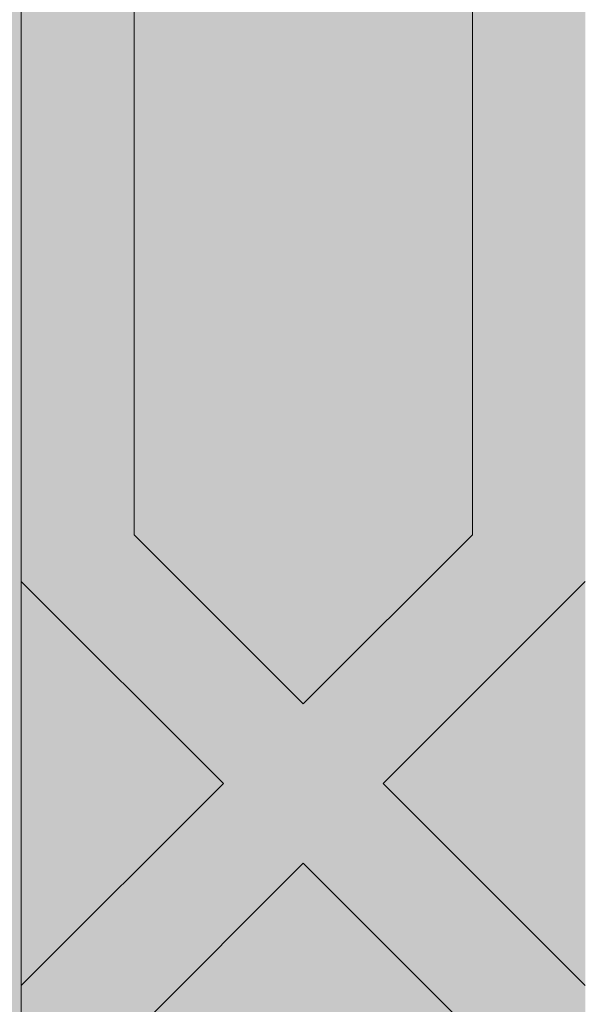
# Model space of a CAD drawing. Units: inches. Extents: x 844 to 2234, y 346 to 1084.
# Tile 78 of 93: x 1997.478 to 1998.757, y 706.514 to 708.742. Entities that reach past the tile are written whole.
import ezdxf

# ---------------------------------------------------------------- set-up
doc = ezdxf.new("R2010")
doc.units = ezdxf.units.IN
doc.header["$MEASUREMENT"] = 0
for name, color, linetype, lineweight in [('A-ANNO-DIMS', 2, 'Continuous', 18), ('furniture', 8, 'Continuous', 18), ('RA-AP-01$0$INT', 35, 'Continuous', 5)]:
    doc.layers.add(name, color=color, linetype=linetype, lineweight=lineweight)
doc.layers.add('RA-AP-01$0$FURN', color=3, linetype='Continuous')
doc.styles.get("Standard").update_dxf_attribs({"font": 'arial.ttf'})
doc.dimstyles.get("Standard").update_dxf_attribs({"dimtxt": 6, "dimasz": 3, "dimexe": 0.18, "dimexo": 0.0625, "dimgap": 0.09, "dimtad": 0, "dimtih": 1, "dimtoh": 1, "dimdec": 1, "dimzin": 0, "dimdsep": 46, "dimlunit": 3, "dimtxsty": 'Standard', "dimblk": 'ARCHTICK', "dimcen": 0.09, "dimadec": 0, "dimazin": 0, "dimtfac": 1, "dimtdec": 1, "dimtofl": 0, "dimtmove": 0, "dimatfit": 3, "dimfxl": 1, "dimtolj": 1, "dimtzin": 0, "dimarcsym": 0})

# ---------------------------------------------------------------- blocks, each defined once
blk = doc.blocks.new('A$C18D01794')
at = {"layer": 'RA-AP-01$0$INT'}
h = blk.add_hatch(color=256, dxfattribs=at)
h.paths.add_polyline_path([(4.355206456958071, -6.156712009588037), (4.355206456958071, -8.056712009588038), (5.455206456958072, -8.056712009588038), (5.455206456958072, -6.156712009588037)])
h.paths.add_polyline_path([(4.405206456958072, -8.006712009588039), (4.405206456958072, -6.206712009588038), (5.405206456958072, -6.206712009588038), (5.405206456958072, -8.006712009588039)], flags=16)
h = blk.add_hatch(color=256, dxfattribs=at)
h.paths.add_polyline_path([(4.505206456958071, -7.585498806127123), (4.46934859260189, -7.549640941759413), (4.505206456958071, -7.513783077414768), (4.505206456958071, -7.381963272220687), (4.469348592616735, -7.346105407867824), (4.505206456958071, -7.310247543514964), (4.505206456958071, -7.178427738324996), (4.469348592586679, -7.142569873965138), (4.505206456952245, -7.106712009588038), (4.476922185709333, -7.106712009588038), (4.455206456960671, -7.128427738343681), (4.433490728198047, -7.106712009588038), (4.405206456946033, -7.106712009588036), (4.441064321339216, -7.142569873969684), (4.40520645695807, -7.178427738362358), (4.405206456958072, -7.310247543472698), (4.441064321364728, -7.346105407867826), (4.40520645695807, -7.381963272262947), (4.40520645695807, -7.513783077378263), (4.441064321354429, -7.549640941786153), (4.405206456958072, -7.585498806170974), (4.405206456958072, -7.717318611286652), (4.441064321333084, -7.753176475673194), (4.405206456958072, -7.789034340036673), (4.405206456958072, -8.006712009588039), (4.644348592588106, -8.006712009588039), (4.680206456964639, -7.970854145211967), (4.716064321341165, -8.006712009588039), (4.869348592586113, -8.006712009588039), (4.905206456964143, -7.970854145210465), (4.941064321342174, -8.006712009588039), (5.094348592587118, -8.006712009588037), (5.130206456963649, -7.970854145211967), (5.166064321340178, -8.006712009588039), (5.405206456958072, -8.006712009588039), (5.405206456958072, -7.789034340024526), (5.369348592595202, -7.753176475673196), (5.40520645695807, -7.717318611298797), (5.40520645695807, -7.585498806158829), (5.369348592573859, -7.549640941786151), (5.40520645695807, -7.51378307739041), (5.40520645695807, -7.381963272250803), (5.36934859256356, -7.346105407867824), (5.405206456958072, -7.310247543484846), (5.405206456958072, -7.178427738350217), (5.369348592589068, -7.142569873969682), (5.405206456982249, -7.106712009588038), (5.376922185730244, -7.106712009588038), (5.355206456967613, -7.128427738343679), (5.333490728218955, -7.10671200958804), (5.305206456976043, -7.106712009588042), (5.341064321341609, -7.142569873965136), (5.305206456958072, -7.178427738337141), (5.305206456958072, -7.310247543502816), (5.34106432131155, -7.346105407867824), (5.305206456958072, -7.381963272232832), (5.30520645695807, -7.513783077402624), (5.341064321326395, -7.549640941759413), (5.305206456958072, -7.585498806139263), (5.305206456958072, -7.717318611299605), (5.341064321347738, -7.753176475677737), (5.305206456958072, -7.78903434007894), (5.30520645695807, -7.906712009588039), (5.166064321336834, -7.906712009588039), (5.130206456963647, -7.942569873961684), (5.094348592590464, -7.906712009588039), (4.941064321338827, -7.906712009588041), (4.905206456964145, -7.942569873963183), (4.869348592589459, -7.906712009588039), (4.716064321337822, -7.906712009588041), (4.680206456964641, -7.942569873961684), (4.644348592591453, -7.906712009588039), (4.505206456958071, -7.906712009588039), (4.505206456958071, -7.789034340066795), (4.469348592580545, -7.753176475677738), (4.505206456958071, -7.717318611311748)])
h.paths.add_polyline_path([(4.485206456974132, -7.709034340046354), (4.45520645695909, -7.739034340051736), (4.425206456974128, -7.709034340057131), (4.425206456993394, -7.593783077384998), (4.45520645699153, -7.563783077396511), (4.485206456993396, -7.593783077408017)], flags=16)
h.paths.add_polyline_path([(4.455206456954537, -7.767318611299197), (4.485206456958242, -7.797318611312542), (4.48520645695951, -7.912569873958716), (4.45520645695415, -7.942569873954422), (4.425206456957888, -7.912569873967813), (4.425206456957888, -7.797318611286197)], flags=16)
h.paths.add_polyline_path([(4.455206456964794, -7.535498806149051), (4.42520645696469, -7.5054988061393), (4.425206456983954, -7.390247543486406), (4.455206456990734, -7.360247543489279), (4.485206456983953, -7.39024754349214), (4.485206456964687, -7.505498806158811)], flags=16)
h.paths.add_polyline_path([(4.499348592588947, -7.926712009585049), (4.636064321340932, -7.926712009585049), (4.666064321342317, -7.956712009586821), (4.636064321343707, -7.986712009585048), (4.499348592575121, -7.986712009585048), (4.469348592591685, -7.956712009591957)], flags=16)
h.paths.add_polyline_path([(4.425206456957888, -7.940854145195974), (4.471064321332215, -7.986712009585049), (4.425206456957888, -7.986712009585049)], flags=16)
h.paths.add_polyline_path([(4.455206456990734, -7.331963272246367), (4.425206456989053, -7.301963272254337), (4.425206456969784, -7.186712009596224), (4.455206456965226, -7.156712009591144), (4.485206456969787, -7.186712009586051), (4.485206456989053, -7.301963272238404)], flags=16)
h.paths.add_polyline_path([(4.72434859258714, -7.926712009586255), (4.861064321340141, -7.926712009586248), (4.891064321340324, -7.956712009586823), (4.861064321340513, -7.986712009586252), (4.724348592586768, -7.986712009586252), (4.694348592586956, -7.956712009586821)], flags=16)
h.paths.add_polyline_path([(4.919348592587961, -7.956712009586821), (4.949348592588145, -7.92671200958625), (5.08606432134115, -7.926712009586253), (5.116064321341327, -7.956712009586823), (5.086064321341519, -7.986712009586252), (4.949348592587774, -7.986712009586252)], flags=16)
h.paths.add_polyline_path([(5.144348592585967, -7.956712009586823), (5.174348592587358, -7.926712009585049), (5.311064321339338, -7.926712009585049), (5.3410643213366, -7.956712009591957), (5.311064321353163, -7.986712009585048), (5.174348592584576, -7.986712009585048)], flags=16)
h.paths.add_polyline_path([(5.32520645693489, -7.593783077408021), (5.355206456936755, -7.563783077396511), (5.385206456934894, -7.593783077384998), (5.38520645695416, -7.709034340057128), (5.355206456969194, -7.739034340051736), (5.325206456954153, -7.709034340046352)], flags=16)
h.paths.add_polyline_path([(5.325206456970042, -7.797318611312542), (5.355206456973747, -7.767318611299197), (5.385206456970398, -7.7973186112862), (5.385206456970398, -7.912569873967816), (5.355206456974136, -7.942569873954422), (5.325206456968778, -7.912569873958716)], flags=16)
h.paths.add_polyline_path([(5.325206456963599, -7.505498806158811), (5.325206456944333, -7.39024754349214), (5.355206456937552, -7.360247543489279), (5.385206456944332, -7.39024754348641), (5.385206456963596, -7.505498806139303), (5.355206456963492, -7.53549880614905)], flags=16)
h.paths.add_polyline_path([(5.32520645693923, -7.301963272238403), (5.3252064569585, -7.186712009586051), (5.355206456963062, -7.156712009591142), (5.3852064569585, -7.186712009596224), (5.385206456939234, -7.301963272254338), (5.355206456937552, -7.331963272246369)], flags=16)
h.paths.add_polyline_path([(5.339348592596071, -7.986712009585048), (5.385206456970398, -7.940854145195972), (5.385206456970396, -7.986712009585048)], flags=16)
h = blk.add_hatch(color=256, dxfattribs=at)
h.paths.add_polyline_path([(4.469348592586677, -7.142569873965136), (4.505206456958073, -7.178427738324996), (4.505206456958071, -7.106712009582215)])
h.paths.add_polyline_path([(4.455206456960671, -7.128427738343681), (4.476922185709333, -7.106712009588038), (4.433490728198045, -7.106712009588038)])
h.paths.add_polyline_path([(4.405206456958073, -7.178427738362358), (4.441064321339218, -7.142569873969684), (4.40520645695807, -7.106712009600073)])
h.paths.add_polyline_path([(4.425206456989053, -7.301963272254335), (4.455206456990736, -7.331963272246371), (4.485206456989055, -7.301963272238399), (4.48520645696979, -7.186712009586054), (4.455206456965227, -7.15671200959114), (4.425206456969784, -7.186712009596224)])
h.paths.add_polyline_path([(4.505206456958073, -7.381963272220689), (4.505206456958071, -7.310247543514961), (4.469348592616738, -7.346105407867826)])
h.paths.add_polyline_path([(4.425206456964688, -7.5054988061393), (4.455206456964794, -7.535498806149051), (4.485206456964689, -7.505498806158811), (4.485206456983951, -7.390247543492138), (4.455206456990736, -7.360247543489277), (4.425206456983956, -7.39024754348641)])
h.paths.add_polyline_path([(4.425206456974126, -7.709034340057128), (4.455206456959092, -7.739034340051736), (4.485206456974132, -7.709034340046356), (4.485206456993396, -7.593783077408017), (4.45520645699153, -7.563783077396511), (4.425206456993394, -7.593783077384999)])
h.paths.add_polyline_path([(4.46934859260189, -7.549640941759415), (4.505206456958071, -7.585498806127123), (4.505206456958073, -7.513783077414766)])
h.paths.add_polyline_path([(4.405206456958073, -7.585498806170972), (4.441064321354427, -7.549640941786151), (4.405206456958072, -7.513783077378263)])
h.paths.add_polyline_path([(4.405206456958072, -7.789034340036673), (4.441064321333084, -7.753176475673194), (4.405206456958072, -7.71731861128665)])
h.paths.add_polyline_path([(4.469348592580547, -7.75317647567774), (4.505206456958071, -7.789034340066795), (4.505206456958071, -7.717318611311744)])
h.paths.add_polyline_path([(4.425206456957888, -7.912569873967814), (4.45520645695415, -7.942569873954422), (4.485206456959507, -7.912569873958718), (4.48520645695824, -7.797318611312542), (4.455206456954537, -7.767318611299197), (4.425206456957888, -7.797318611286202)])
h.paths.add_polyline_path([(4.425206456957888, -7.986712009585049), (4.471064321332215, -7.986712009585049), (4.425206456957888, -7.940854145195972)])
h.paths.add_polyline_path([(4.499348592575121, -7.986712009585048), (4.636064321343707, -7.986712009585049), (4.666064321342317, -7.956712009586823), (4.636064321340932, -7.926712009585049), (4.499348592588945, -7.926712009585049), (4.469348592591685, -7.95671200959196)])
h.paths.add_polyline_path([(4.680206456964641, -7.942569873961684), (4.716064321337824, -7.906712009588039), (4.644348592591454, -7.906712009588039)])
h.paths.add_polyline_path([(4.644348592588108, -8.006712009588039), (4.716064321341167, -8.006712009588039), (4.680206456964637, -7.970854145211964)])
h.paths.add_polyline_path([(4.724348592586768, -7.98671200958625), (4.861064321340514, -7.986712009586252), (4.891064321340324, -7.956712009586819), (4.861064321340141, -7.92671200958625), (4.724348592587134, -7.926712009586255), (4.694348592586957, -7.956712009586821)])
h.paths.add_polyline_path([(4.905206456964143, -7.942569873963183), (4.941064321338827, -7.906712009588039), (4.869348592589457, -7.906712009588037)])
h.paths.add_polyline_path([(4.869348592586113, -8.006712009588039), (4.941064321342172, -8.006712009588037), (4.905206456964145, -7.970854145210463)])
h.paths.add_polyline_path([(4.949348592587774, -7.986712009586252), (5.086064321341521, -7.986712009586252), (5.116064321341329, -7.956712009586823), (5.08606432134115, -7.926712009586253), (4.949348592588145, -7.92671200958625), (4.919348592587961, -7.956712009586819)])
h.paths.add_polyline_path([(5.130206456963645, -7.942569873961684), (5.166064321336834, -7.906712009588039), (5.094348592590464, -7.906712009588039)])
h.paths.add_polyline_path([(5.094348592587119, -8.006712009588039), (5.166064321340178, -8.006712009588039), (5.130206456963651, -7.970854145211967)])
h.paths.add_polyline_path([(5.174348592584578, -7.986712009585048), (5.311064321353163, -7.986712009585048), (5.341064321336602, -7.956712009591958), (5.31106432133934, -7.926712009585049), (5.174348592587352, -7.926712009585049), (5.144348592585969, -7.956712009586823)])
h.paths.add_polyline_path([(5.325206456968778, -7.912569873958718), (5.355206456974136, -7.942569873954422), (5.385206456970396, -7.912569873967814), (5.385206456970396, -7.797318611286199), (5.355206456973747, -7.767318611299197), (5.325206456970044, -7.797318611312544)])
h.paths.add_polyline_path([(5.339348592596073, -7.986712009585048), (5.385206456970396, -7.986712009585049), (5.385206456970398, -7.94085414519597)])
h.paths.add_polyline_path([(5.325206456954155, -7.709034340046354), (5.355206456969194, -7.739034340051734), (5.38520645695416, -7.709034340057128), (5.385206456934896, -7.593783077384999), (5.355206456936758, -7.563783077396513), (5.325206456934888, -7.593783077408019)])
h.paths.add_polyline_path([(5.305206456958072, -7.789034340078938), (5.341064321347739, -7.753176475677738), (5.305206456958072, -7.717318611299605)])
h.paths.add_polyline_path([(5.369348592595204, -7.753176475673194), (5.40520645695807, -7.789034340024526), (5.405206456958072, -7.717318611298798)])
h.paths.add_polyline_path([(5.405206456958072, -7.585498806158831), (5.405206456958072, -7.513783077390407), (5.369348592573857, -7.549640941786151)])
h.paths.add_polyline_path([(5.305206456958072, -7.585498806139266), (5.341064321326393, -7.549640941759413), (5.305206456958072, -7.513783077402626)])
h.paths.add_polyline_path([(5.325206456963599, -7.50549880615881), (5.355206456963494, -7.535498806149055), (5.385206456963598, -7.505498806139302), (5.385206456944334, -7.390247543486411), (5.355206456937552, -7.360247543489279), (5.325206456944333, -7.39024754349214)])
h.paths.add_polyline_path([(5.305206456958072, -7.38196327223283), (5.341064321311551, -7.346105407867824), (5.305206456958072, -7.31024754350282)])
h.paths.add_polyline_path([(5.325206456939231, -7.301963272238404), (5.355206456937552, -7.331963272246369), (5.385206456939235, -7.301963272254335), (5.385206456958502, -7.186712009596224), (5.355206456963061, -7.156712009591142), (5.3252064569585, -7.186712009586051)])
h.paths.add_polyline_path([(5.404581768715993, -7.381338584008926, -0.001217816984214), (5.405206456958072, -7.381112009582329), (5.405206456958072, -7.310247543484846), (5.369348592563558, -7.346105407867826)])
h.paths.add_polyline_path([(5.36934859258907, -7.142569873969684), (5.40520645695807, -7.178427738350215), (5.405206456958072, -7.106712009612218)])
h.paths.add_polyline_path([(5.355206456967613, -7.128427738343683), (5.376922185730239, -7.106712009588038), (5.333490728218953, -7.10671200958804)])
h.paths.add_polyline_path([(5.30520645695807, -7.178427738337139), (5.341064321341609, -7.142569873965134), (5.305206456958074, -7.10671200957007)])
for p, q in [((5.325206456963599, -7.505498806158811), (5.35520645696349, -7.535498806149051)), ((5.385206456963598, -7.5054988061393), (5.35520645696349, -7.535498806149051)), ((5.305206456959569, -7.513783077404122), (5.341064321342035, -7.549640941775054)), ((5.405206456959569, -7.513783077388909), (5.369348592589498, -7.54964094177051)), ((5.305206456939818, -7.58549880615752), (5.341064321310754, -7.549640941775056)), ((5.405206456939818, -7.585498806140577), (5.369348592558215, -7.549640941770508)), ((5.32520645693489, -7.593783077408017), (5.355206456936756, -7.563783077396511)), ((5.385206456934892, -7.593783077384996), (5.355206456936756, -7.563783077396511)), ((5.32520645693489, -7.593783077408017), (5.325206456954155, -7.709034340046354)), ((5.385206456934892, -7.593783077384996), (5.385206456954159, -7.709034340057129))]:
    blk.add_line(p, q, dxfattribs=at)
blk.add_lwpolyline([(5.405206456958072, -7.106712009588038), (5.405206456958072, -8.006712009588039)], dxfattribs=at)
blk = doc.blocks.new('A$C5D2F253E')
at = {"layer": 'RA-AP-01$0$FURN', "xscale": -0.7999999999883585, "yscale": 0.7999999999883585, "zscale": 0.8, "rotation": 90}
blk.add_blockref('A$C18D01794', (-5.687757199772477, 4.75791982714071), dxfattribs=at)
blk = doc.blocks.new('_ArchTick')
at = {"color": 0, "linetype": 'ByBlock', "const_width": 0.15}
blk.add_lwpolyline([(-0.5, -0.5), (0.5, 0.5)], dxfattribs=at)
blk = doc.blocks.new('*D121')
at = {"layer": 'A-ANNO-DIMS', "color": 0, "lineweight": -2, "transparency": 16777216}
for p, q in [((2030.271987351997, 734.262611118704), (2040.245275089302, 734.262611118704)), ((2040.065275089302, 734.262611118704), (2040.065275089302, 704.6043509484256)), ((2040.065275089302, 668.557359536674), (2040.065275089302, 698.2156197069523)), ((2030.271987351997, 668.557359536674), (2040.245275089302, 668.557359536674))]:
    blk.add_line(p, q, dxfattribs=at)
at = {"layer": 'Defpoints', "color": 0, "transparency": 16777216}
for p in [(2030.209487351997, 734.262611118704), (2040.065275089302, 734.262611118704), (2030.209487351997, 668.557359536674)]:
    blk.add_point(p, dxfattribs=at)
at = {"layer": 'A-ANNO-DIMS', "color": 0, "lineweight": -2, "transparency": 16777216, "xscale": 3, "yscale": 3, "zscale": 3}
for p, rotation in [((2040.065275089302, 734.262611118704), 90), ((2040.065275089302, 668.557359536674), 270)]:
    blk.add_blockref('_ArchTick', p, dxfattribs=dict(at, rotation=rotation))
at = {"layer": 'A-ANNO-DIMS', "color": 0, "transparency": 16777216, "insert": (2040.065275089302, 701.4099853276883), "char_height": 6, "attachment_point": 5}
blk.add_mtext('\\A1;LOUNGE SET 5\'-5 1/2" TYP.', dxfattribs=at)

msp = doc.modelspace()

# ---------------------------------------------------------------- block references
at = {"layer": 'furniture', "xscale": -15.94108302203742, "yscale": 15.94108302203742, "zscale": 15.94108302203742, "rotation": 270}
msp.add_blockref('A$C5D2F253E', (1990.567271852805, 701.4028671565849), dxfattribs=at)

# ---------------------------------------------------------------- dimensions: what is measured, and where the dimension line sits
at = {"layer": 'A-ANNO-DIMS'}
dim = msp.add_linear_dim(base=(2040.065275089302, 734.262611118704), p1=(2030.209487351996, 668.5573595366737), p2=(2030.209487351996, 734.2626111187037), angle=90, text='LOUNGE SET <> TYP.', dimstyle='Standard', override={"dimdec": 1, "dimlfac": 1, "dimrnd": 0, "dimzin": 1, "dimdsep": 46, "dimlunit": 4, "dimfrac": 2}, dxfattribs=at)
dim.commit()
dim.dimension.update_dxf_attribs({"geometry": '*D121', "text_midpoint": (2040.065275089302, 701.4099853276883)})

doc.saveas('drawing.dxf')
